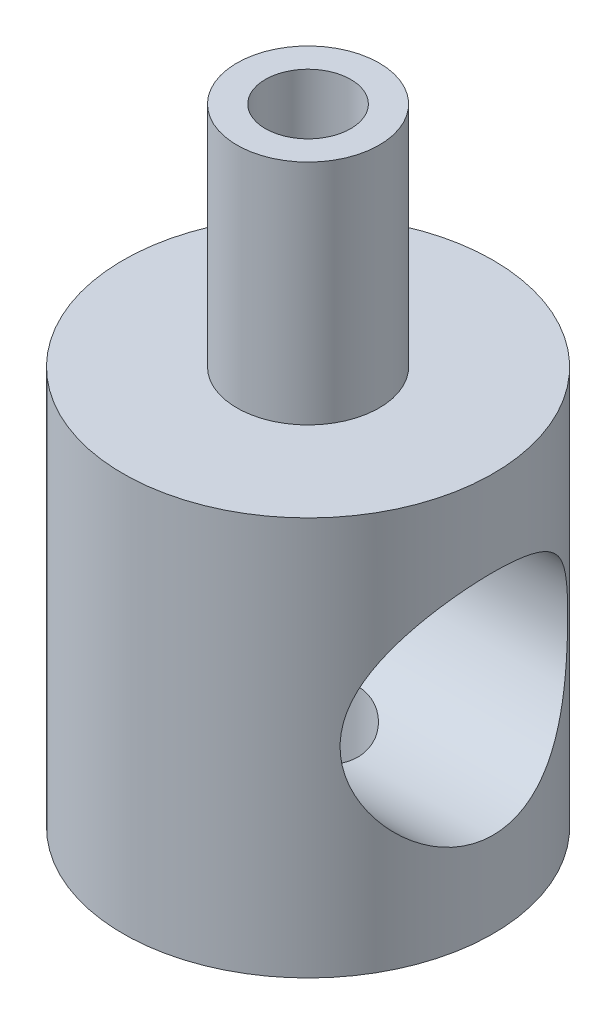
SolidWorks part; units mm, degrees
material "Plain Carbon Steel"
ref_plane "Front Plane" through (0, 0, 0) normal (0, 0, 1) x (1, 0, 0)
ref_plane "Top Plane" through (0, 0, 0) normal (0, 1, 0) x (1, 0, 0)
ref_plane "Right Plane" through (0, 0, 0) normal (1, 0, 0) x (0, 0, -1)
sketch "Barrel Profile Sketch" plane through (0, 0, 0) normal (0, 0, 1) x (1, 0, 0)
  line L0 (0, 0) -> (0, 22)
  line L1 (0, 22) -> (2.5, 22)
  line L2 (2.5, 22) -> (2.5, 14)
  line L3 (2.5, 14) -> (6.5, 14)
  line L4 (6.5, 14) -> (6.5, 0)
  line L5 (6.5, 0) -> (0, 0)
  dimension "D1" = 2.5
  dimension "D2" = 6.5
  dimension "D3" = 8
  dimension "D4" = 22
revolve "Barrel Body Revolve" add sketch "Barrel Profile Sketch" angle 360 about L0
sketch "Cross Hole Sketch" plane through (0, 0, 0) normal (1, 0, 0) x (0, 0, -1)
  circle A0 centre (0, 7) radius 4
  dimension "D1" = 8
  dimension "D2" = 7
extrude "Cross Hole Ø8" cut sketch "Cross Hole Sketch" against normal mid plane 88
sketch "Nipple Pocket Sketch" plane through (0, 0, 0) normal (0, -1, 0) x (1, 0, 0)
  circle A0 centre (0, 0) radius 1.75
  dimension "D1" = 3.5
extrude "Nipple Pocket Ø3.5" cut sketch "Nipple Pocket Sketch" against normal blind 5
sketch "Cable Bore Sketch" plane through (0, 22, 0) normal (0, 1, 0) x (1, 0, 0)
  circle A0 centre (0, 0) radius 1.5
  dimension "D1" = 3
extrude "Cable Bore Ø3" cut sketch "Cable Bore Sketch" against normal blind 13
